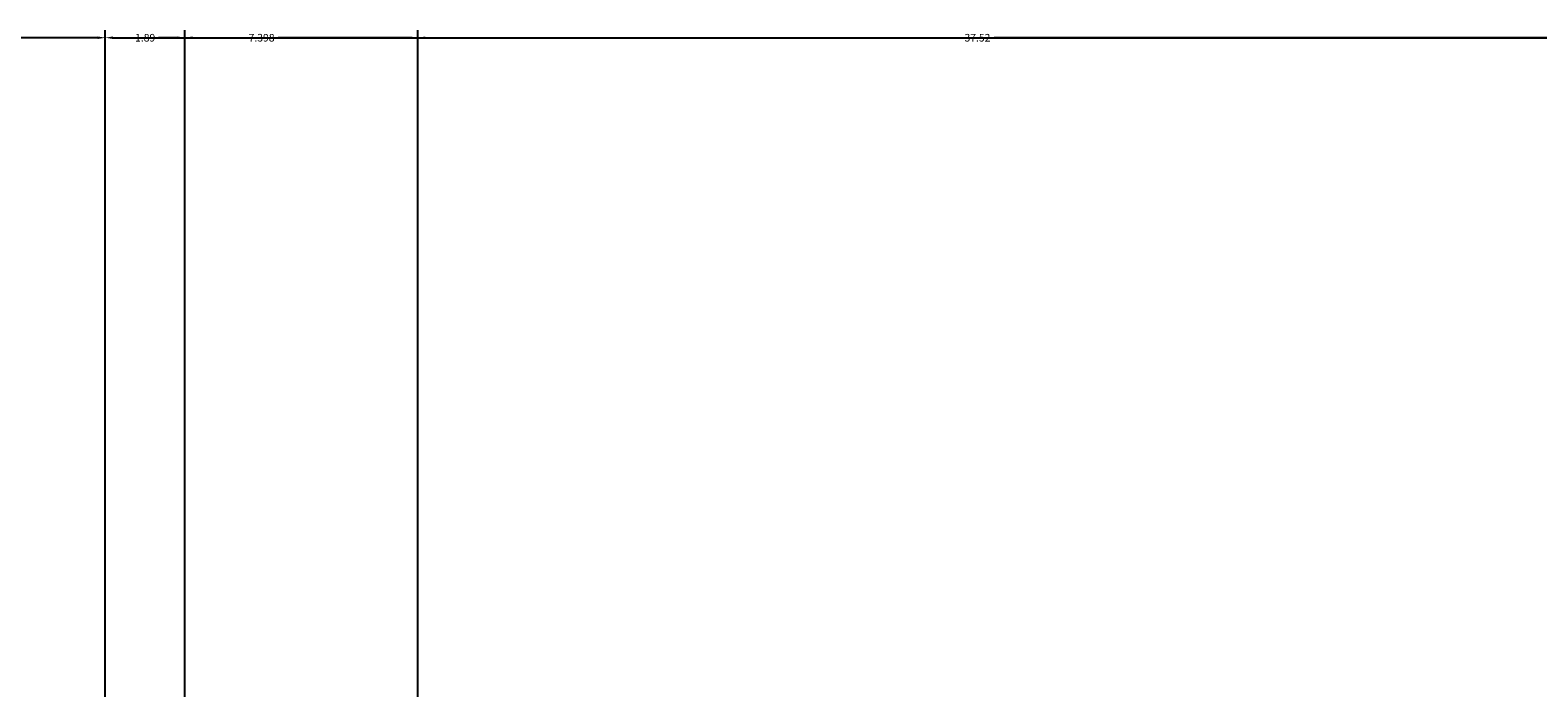
# Model space of a CAD drawing. Units: feet. Extents: x 2695 to 2912, y 795 to 1139.
# Tile 72 of 83: x 2769 to 2805, y 1123 to 1139. Entities that reach past the tile are written whole.
import ezdxf

# ---------------------------------------------------------------- set-up
doc = ezdxf.new("R2010")
doc.units = ezdxf.units.FT
doc.layers.add('A-ANNO-DIMS', color=2, linetype='Continuous', lineweight=18)
doc.styles.get("Standard").update_dxf_attribs({"font": 'arial.ttf'})
doc.dimstyles.get("Standard").update_dxf_attribs({"dimtxt": 0.18, "dimasz": 0.18, "dimexe": 0.18, "dimexo": 0.0625, "dimgap": 0.09, "dimtad": 0, "dimtih": 1, "dimtoh": 1, "dimdec": 1, "dimzin": 0, "dimdsep": 46, "dimlunit": 3, "dimtxsty": 'Standard', "dimcen": 0.09, "dimadec": 0, "dimazin": 0, "dimtfac": 1, "dimtdec": 1, "dimtofl": 0, "dimtmove": 0, "dimatfit": 3, "dimfxl": 1, "dimtolj": 1, "dimtzin": 0, "dimarcsym": 0})

# ---------------------------------------------------------------- blocks, each defined once
blk = doc.blocks.new('*D8')
at = {"layer": 'A-ANNO-DIMS', "color": 0, "lineweight": -2, "transparency": 16777216}
for p, q in [((2715.885, 1050.373), (2715.885, 1138.886)), ((2716.065, 1138.706), (2742.866, 1138.706)), ((2770.456, 1138.706), (2743.655, 1138.706)), ((2770.636, 1122.993), (2770.636, 1138.886))]:
    blk.add_line(p, q, dxfattribs=at)
at = {"layer": 'A-ANNO-DIMS', "color": 0, "transparency": 16777216}
for points in [[(2716.065, 1138.736), (2716.065, 1138.676), (2715.885, 1138.706)], [(2770.456, 1138.736), (2770.456, 1138.676), (2770.636, 1138.706)]]:
    blk.add_solid(points, dxfattribs=at)
at = {"layer": 'Defpoints', "color": 0, "transparency": 16777216}
for p in [(2770.636, 1138.706), (2770.636, 1122.931), (2715.885, 1050.311)]:
    blk.add_point(p, dxfattribs=at)
at = {"layer": 'A-ANNO-DIMS', "color": 0, "transparency": 16777216, "insert": (2743.261, 1138.706), "char_height": 0.18, "attachment_point": 5}
blk.add_mtext('\\A1;54.75', dxfattribs=at)
blk = doc.blocks.new('*D9')
at = {"layer": 'A-ANNO-DIMS', "color": 0, "lineweight": -2, "transparency": 16777216}
for p, q in [((2770.636, 1122.993), (2770.636, 1138.886)), ((2770.816, 1138.706), (2773.942, 1138.706)), ((2777.854, 1138.706), (2774.728, 1138.706)), ((2778.034, 1020.886), (2778.034, 1138.886))]:
    blk.add_line(p, q, dxfattribs=at)
at = {"layer": 'A-ANNO-DIMS', "color": 0, "transparency": 16777216}
for points in [[(2770.816, 1138.736), (2770.816, 1138.676), (2770.636, 1138.706)], [(2777.854, 1138.736), (2777.854, 1138.676), (2778.034, 1138.706)]]:
    blk.add_solid(points, dxfattribs=at)
at = {"layer": 'Defpoints', "color": 0, "transparency": 16777216}
for p in [(2778.034, 1138.706), (2770.636, 1122.931), (2778.034, 1020.824)]:
    blk.add_point(p, dxfattribs=at)
at = {"layer": 'A-ANNO-DIMS', "color": 0, "transparency": 16777216, "insert": (2774.335, 1138.706), "char_height": 0.18, "attachment_point": 5}
blk.add_mtext('\\A1;7.398', dxfattribs=at)
blk = doc.blocks.new('*D10')
at = {"layer": 'A-ANNO-DIMS', "color": 0, "lineweight": -2, "transparency": 16777216}
for p, q in [((2778.034, 1020.886), (2778.034, 1138.886)), ((2778.214, 1138.706), (2810.411, 1138.706)), ((2843.395, 1138.706), (2811.198, 1138.706)), ((2843.575, 1020.886), (2843.575, 1138.886))]:
    blk.add_line(p, q, dxfattribs=at)
at = {"layer": 'A-ANNO-DIMS', "color": 0, "transparency": 16777216}
for points in [[(2778.214, 1138.736), (2778.214, 1138.676), (2778.034, 1138.706)], [(2843.395, 1138.736), (2843.395, 1138.676), (2843.575, 1138.706)]]:
    blk.add_solid(points, dxfattribs=at)
at = {"layer": 'Defpoints', "color": 0, "transparency": 16777216}
for p in [(2843.575, 1138.706), (2778.034, 1020.824), (2843.575, 1020.824)]:
    blk.add_point(p, dxfattribs=at)
at = {"layer": 'A-ANNO-DIMS', "color": 0, "transparency": 16777216, "insert": (2810.805, 1138.706), "char_height": 0.18, "attachment_point": 5}
blk.add_mtext('\\A1;65.54', dxfattribs=at)
blk = doc.blocks.new('*D48')
at = {"layer": 'A-ANNO-DIMS', "color": 0, "lineweight": -2, "transparency": 16777216}
for p, q in [((2770.636, 972.03), (2770.636, 1138.886)), ((2770.816, 1138.706), (2771.263, 1138.706)), ((2772.342, 1138.706), (2771.894, 1138.706)), ((2772.522, 972.03), (2772.522, 1138.886))]:
    blk.add_line(p, q, dxfattribs=at)
at = {"layer": 'A-ANNO-DIMS', "color": 0, "transparency": 16777216}
for points in [[(2770.816, 1138.736), (2770.816, 1138.676), (2770.636, 1138.706)], [(2772.342, 1138.736), (2772.342, 1138.676), (2772.522, 1138.706)]]:
    blk.add_solid(points, dxfattribs=at)
at = {"layer": 'Defpoints', "color": 0, "transparency": 16777216}
for p in [(2772.522, 1138.706), (2770.636, 971.967), (2772.522, 971.967)]:
    blk.add_point(p, dxfattribs=at)
at = {"layer": 'A-ANNO-DIMS', "color": 0, "transparency": 16777216, "insert": (2771.579, 1138.706), "char_height": 0.18, "attachment_point": 5}
blk.add_mtext('\\A1;1.89', dxfattribs=at)
blk = doc.blocks.new('*D49')
at = {"layer": 'A-ANNO-DIMS', "color": 0, "lineweight": -2, "transparency": 16777216}
for p, q in [((2772.522, 972.03), (2772.522, 1138.886)), ((2772.702, 1138.706), (2790.888, 1138.706)), ((2809.861, 1138.706), (2791.674, 1138.706)), ((2810.041, 972.03), (2810.041, 1138.886))]:
    blk.add_line(p, q, dxfattribs=at)
at = {"layer": 'A-ANNO-DIMS', "color": 0, "transparency": 16777216}
for points in [[(2772.702, 1138.736), (2772.702, 1138.676), (2772.522, 1138.706)], [(2809.861, 1138.736), (2809.861, 1138.676), (2810.041, 1138.706)]]:
    blk.add_solid(points, dxfattribs=at)
at = {"layer": 'Defpoints', "color": 0, "transparency": 16777216}
for p in [(2810.041, 1138.706), (2772.522, 971.967), (2810.041, 971.967)]:
    blk.add_point(p, dxfattribs=at)
at = {"layer": 'A-ANNO-DIMS', "color": 0, "transparency": 16777216, "insert": (2791.281, 1138.706), "char_height": 0.18, "attachment_point": 5}
blk.add_mtext('\\A1;37.52', dxfattribs=at)

msp = doc.modelspace()

# ---------------------------------------------------------------- dimensions: what is measured, and where the dimension line sits
at = {"layer": 'A-ANNO-DIMS'}
for base, p1, p2, override, picture, middle in [((2770.6361, 1138.7056), (2715.8852, 1050.3105), (2770.6361, 1122.9306), {"dimdec": 2, "dimlfac": 1, "dimrnd": 0, "dimzin": 0, "dimdsep": 46, "dimlunit": 2}, '*D8', (2743.2606, 1138.7056)), ((2778.0341, 1138.7056), (2770.6361, 1122.9306), (2778.0341, 1020.8235), {"dimdec": 3, "dimlfac": 1, "dimrnd": 0, "dimzin": 0, "dimdsep": 46, "dimlunit": 2}, '*D9', (2774.3351, 1138.7056)), ((2772.5216, 1138.7056), (2770.6361, 971.9673), (2772.5216, 971.9673), {"dimdec": 2, "dimlfac": 1, "dimrnd": 0, "dimzin": 0, "dimdsep": 46, "dimlunit": 2}, '*D48', (2771.5788, 1138.7056)), ((2810.0407, 1138.7056), (2772.5216, 971.9673), (2810.0407, 971.9673), {"dimdec": 2, "dimlfac": 1, "dimrnd": 0, "dimzin": 0, "dimdsep": 46, "dimlunit": 2}, '*D49', (2791.2811, 1138.7056)), ((2843.575, 1138.7056), (2778.0341, 1020.8235), (2843.575, 1020.8235), {"dimdec": 2, "dimlfac": 1, "dimrnd": 0, "dimzin": 0, "dimdsep": 46, "dimlunit": 2}, '*D10', (2810.8045, 1138.7056))]:
    dim = msp.add_linear_dim(base=base, p1=p1, p2=p2, dimstyle='Standard', override=override, dxfattribs=at)
    dim.commit()
    dim.dimension.update_dxf_attribs({"geometry": picture, "text_midpoint": middle})

doc.saveas('drawing.dxf')
